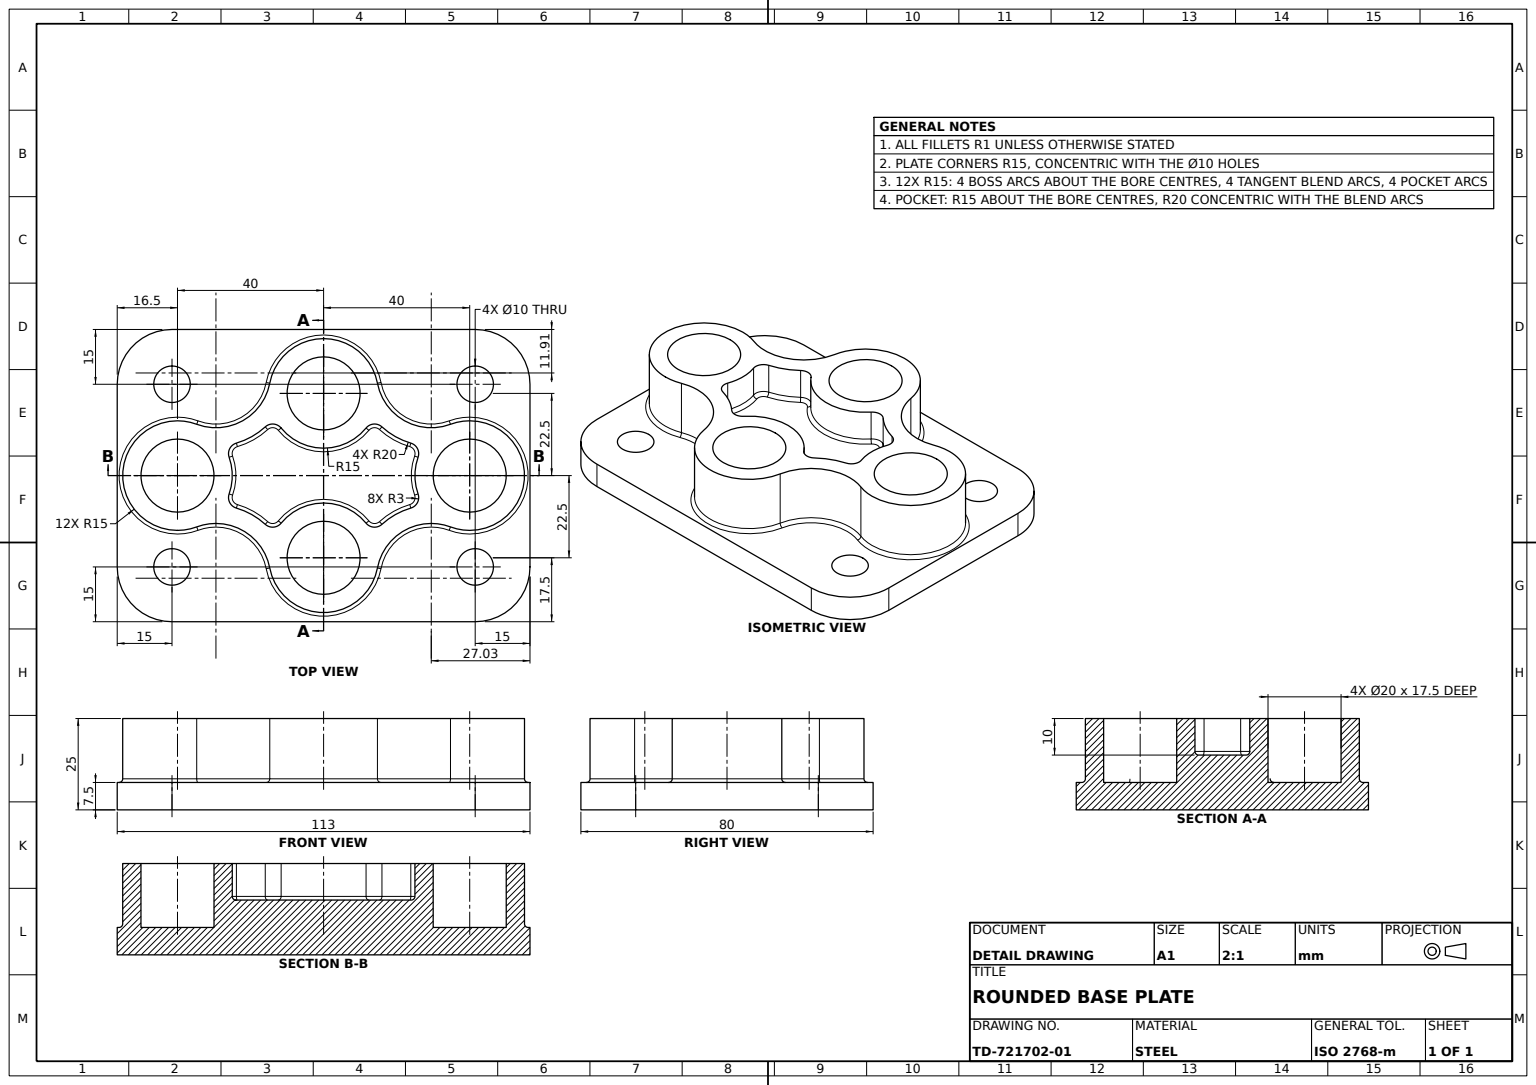
SolidWorks part; units mm, degrees
material "Plain Carbon Steel"
ref_plane "Front Plane" through (0, 0, 0) normal (0, 0, 1) x (1, 0, 0)
ref_plane "Top Plane" through (0, 0, 0) normal (0, 1, 0) x (1, 0, 0)
ref_plane "Right Plane" through (0, 0, 0) normal (1, 0, 0) x (0, 0, -1)
sketch "Base Plate Sketch" plane through (0, 0, 0) normal (0, 1, 0) x (1, 0, 0)
  line L0 (0, 68.9409) -> (0, -55.7389) construction
  line L1 (-56.5, -40) -> (56.5, -40)
  line L2 (-56.5, -40) -> (-56.5, 40)
  line L3 (-56.5, 40) -> (56.5, 40)
  line L4 (56.5, -40) -> (56.5, 40)
  line L5 (-56.5, -40) -> (56.5, 40) construction
  line L6 (-56.5, 40) -> (56.5, -40) construction
  line L7 (135.8746, 0) -> (-84.5878, 0) construction
  point P0 (0, 0)
  dimension "D1" = 80
  dimension "D2" = 113
extrude "Base Plate 113x80x7.5" add sketch "Base Plate Sketch" against normal blind 7.5
sketch "Quad Boss Profile Sketch" plane through (0, 0, 0) normal (0, 1, 0) x (1, 0, 0)
  line L0 (0, 43.4114) -> (0, -48.2823) construction
  line L1 (-74.7675, 0) -> (72.0885, 0) construction
  arc A0 (-34.737, 14.0464) -> (-34.737, -14.0464) centre (-40, 0) ccw
  circle A1 centre (-40, 0) radius 10
  circle A2 centre (0, -22.5) radius 10
  arc A3 (-14.737, -25.2964) -> (14.737, -25.2964) centre (0, -22.5) ccw
  circle A4 centre (40, 0) radius 10
  arc A5 (25.8616, -5.0107) -> (25.8616, 5.0107) centre (40, 0) cw
  circle A6 centre (0, 22.5) radius 10
  arc A7 (11.624, 13.0194) -> (-11.624, 13.0194) centre (0, 22.5) cw
  arc A8 (-34.737, -14.0464) -> (-14.737, -25.2964) centre (-29.4741, -28.0928) cw
  arc A9 (-23.874, -8.8928) -> (-15.9738, -13.3366) centre (-29.4741, -28.0928) cw
  arc A10 (-11.624, 13.0194) -> (-15.9738, 13.3366) centre (-13.9488, 11.1232) ccw
  arc A11 (-23.874, 8.8928) -> (-25.8616, 5.0107) centre (-23.034, 6.0128) ccw
  arc A12 (-23.874, 8.8928) -> (-15.9738, 13.3366) centre (-29.4741, 28.0928) ccw
  arc A13 (11.624, -13.0194) -> (15.9738, -13.3366) centre (13.9488, -11.1232) ccw
  arc A14 (-34.737, 14.0464) -> (-14.737, 25.2964) centre (-29.4741, 28.0928) ccw
  arc A15 (23.874, -8.8928) -> (25.8616, -5.0107) centre (23.034, -6.0128) ccw
  arc A16 (-23.874, -8.8928) -> (-25.8616, -5.0107) centre (-23.034, -6.0128) cw
  arc A17 (-11.624, -13.0194) -> (-15.9738, -13.3366) centre (-13.9488, -11.1232) cw
  arc A18 (34.737, 14.0464) -> (14.737, 25.2964) centre (29.4741, 28.0928) cw
  arc A19 (34.737, -14.0464) -> (14.737, -25.2964) centre (29.4741, -28.0928) ccw
  arc A20 (23.874, -8.8928) -> (15.9738, -13.3366) centre (29.4741, -28.0928) ccw
  arc A21 (23.874, 8.8928) -> (25.8616, 5.0107) centre (23.034, 6.0128) cw
  arc A22 (11.624, 13.0194) -> (15.9738, 13.3366) centre (13.9488, 11.1232) cw
  arc A23 (23.874, 8.8928) -> (15.9738, 13.3366) centre (29.4741, 28.0928) cw
  arc A24 (11.624, -13.0194) -> (-11.624, -13.0194) centre (0, -22.5) ccw
  arc A25 (34.737, 14.0464) -> (34.737, -14.0464) centre (40, 0) cw
  arc A26 (-14.737, 25.2964) -> (14.737, 25.2964) centre (0, 22.5) cw
  arc A27 (-25.8616, -5.0107) -> (-25.8616, 5.0107) centre (-40, 0) ccw
  dimension "D3" = 15
  dimension "D4" = 20
  dimension "D5" = 3
  dimension "D6" = 15
  dimension "D7" = 20
  dimension "D1" = 40
  dimension "D2" = 22.5
extrude "Quad Boss Body H17.5" add sketch "Quad Boss Profile Sketch" along normal blind 17.5
fillet "Boss Root Fillet R1" radius 1 8 edges at (-55, 0, 0) (-22.1201, 0, -15.0192) (0, 0, -37.5) (22.1201, 0, -15.0192) (55, 0, 0) (22.1201, 0, 15.0192) (0, 0, 37.5) (-22.1201, 0, 15.0192)
fillet "Plate Corner Fillets R15" radius 15 4 edges at (-56.5, -3.75, 40) (-56.5, -3.75, -40) (56.5, -3.75, -40) (56.5, -3.75, 40)
sketch "Bore Cut Sketch" plane through (0, 0, 0) normal (0, 1, 0) x (1, 0, 0)
  line L0 (0, 43.1679) -> (0, -48.6476) construction
  line L1 (78.6642, 0) -> (-74.8892, 0) construction
  line L2 (-56.5, 25) -> (-56.5, -25) construction
  circle A0 centre (-41.5, 25) radius 5
  circle A1 centre (-41.5, -25) radius 5
  circle A2 centre (41.5, -25) radius 5
  circle A3 centre (41.5, 25) radius 5
  dimension "D1" = 10
  dimension "D2" = 10
  dimension "D3" = 25
  dimension "D4" = 15
  dimension "D5" = 15
  dimension "D6" = 25
extrude "Bore Cuts D17.5" cut sketch "Bore Cut Sketch" against normal blind 17.5
sketch "Boss Web Offset Sketch" plane through (0, 0, 0) normal (0, 1, 0) x (1, 0, 0)
  arc A16 (-15.9738, -13.3366) -> (-11.624, -13.0194) centre (-13.9488, -11.1232) ccw
  arc A17 (11.624, -13.0194) -> (-11.624, -13.0194) centre (0, -22.5) ccw
  arc A18 (11.624, -13.0194) -> (15.9738, -13.3366) centre (13.9488, -11.1232) ccw
  arc A19 (23.874, -8.8928) -> (15.9738, -13.3366) centre (29.4741, -28.0928) ccw
  arc A20 (23.874, -8.8928) -> (25.8616, -5.0107) centre (23.034, -6.0128) ccw
  arc A21 (25.8616, 5.0107) -> (25.8616, -5.0107) centre (40, 0) ccw
  arc A22 (25.8616, 5.0107) -> (23.874, 8.8928) centre (23.034, 6.0128) ccw
  arc A23 (15.9738, 13.3366) -> (23.874, 8.8928) centre (29.4741, 28.0928) ccw
  arc A24 (15.9738, 13.3366) -> (11.624, 13.0194) centre (13.9488, 11.1232) ccw
  arc A25 (-11.624, 13.0194) -> (11.624, 13.0194) centre (0, 22.5) ccw
  arc A26 (-11.624, 13.0194) -> (-15.9738, 13.3366) centre (-13.9488, 11.1232) ccw
  arc A27 (-23.874, 8.8928) -> (-15.9738, 13.3366) centre (-29.4741, 28.0928) ccw
  arc A28 (-23.874, 8.8928) -> (-25.8616, 5.0107) centre (-23.034, 6.0128) ccw
  arc A29 (-25.8616, -5.0107) -> (-25.8616, 5.0107) centre (-40, 0) ccw
  arc A30 (-25.8616, -5.0107) -> (-23.874, -8.8928) centre (-23.034, -6.0128) ccw
  arc A31 (-15.9738, -13.3366) -> (-23.874, -8.8928) centre (-29.4741, -28.0928) ccw
  arc A32 (-15.9738, -13.3366) -> (-11.624, -13.0194) centre (-13.9488, -11.1232) ccw
  arc A33 (11.624, -13.0194) -> (-11.624, -13.0194) centre (0, -22.5) ccw
  arc A34 (11.624, -13.0194) -> (15.9738, -13.3366) centre (13.9488, -11.1232) ccw
  arc A35 (23.874, -8.8928) -> (15.9738, -13.3366) centre (29.4741, -28.0928) ccw
  arc A36 (23.874, -8.8928) -> (25.8616, -5.0107) centre (23.034, -6.0128) ccw
  arc A37 (25.8616, 5.0107) -> (25.8616, -5.0107) centre (40, 0) ccw
  arc A38 (25.8616, 5.0107) -> (23.874, 8.8928) centre (23.034, 6.0128) ccw
  arc A39 (15.9738, 13.3366) -> (23.874, 8.8928) centre (29.4741, 28.0928) ccw
  arc A40 (15.9738, 13.3366) -> (11.624, 13.0194) centre (13.9488, 11.1232) ccw
  arc A41 (-11.624, 13.0194) -> (11.624, 13.0194) centre (0, 22.5) ccw
  arc A42 (-11.624, 13.0194) -> (-15.9738, 13.3366) centre (-13.9488, 11.1232) ccw
  arc A43 (-23.874, 8.8928) -> (-15.9738, 13.3366) centre (-29.4741, 28.0928) ccw
  arc A44 (-23.874, 8.8928) -> (-25.8616, 5.0107) centre (-23.034, 6.0128) ccw
  arc A45 (-25.8616, -5.0107) -> (-25.8616, 5.0107) centre (-40, 0) ccw
  arc A46 (-25.8616, -5.0107) -> (-23.874, -8.8928) centre (-23.034, -6.0128) ccw
  arc A47 (-15.9738, -13.3366) -> (-23.874, -8.8928) centre (-29.4741, -28.0928) ccw
  dimension "D1" = 0
extrude "Boss Web H7.5" add sketch "Boss Web Offset Sketch" along normal blind 7.5
fillet "Web Blend Fillet R1" radius 1 16 edges at (0, 7.5, -7.5) (13.7305, 7.5, -14.1153) (19.6688, 7.5, -10.6613) (25.7043, 7.5, -7.38) (25, 7.5, 0) (25.7043, 7.5, 7.38) (19.6688, 7.5, 10.6613) (13.7305, 7.5, 14.1153) (0, 7.5, 7.5) (-13.7305, 7.5, 14.1153) (-19.6688, 7.5, 10.6613) (-25.7043, 7.5, 7.38) (-25, 7.5, 0) (-25.7043, 7.5, -7.38) (-19.6688, 7.5, -10.6613) (-13.7305, 7.5, -14.1153)
